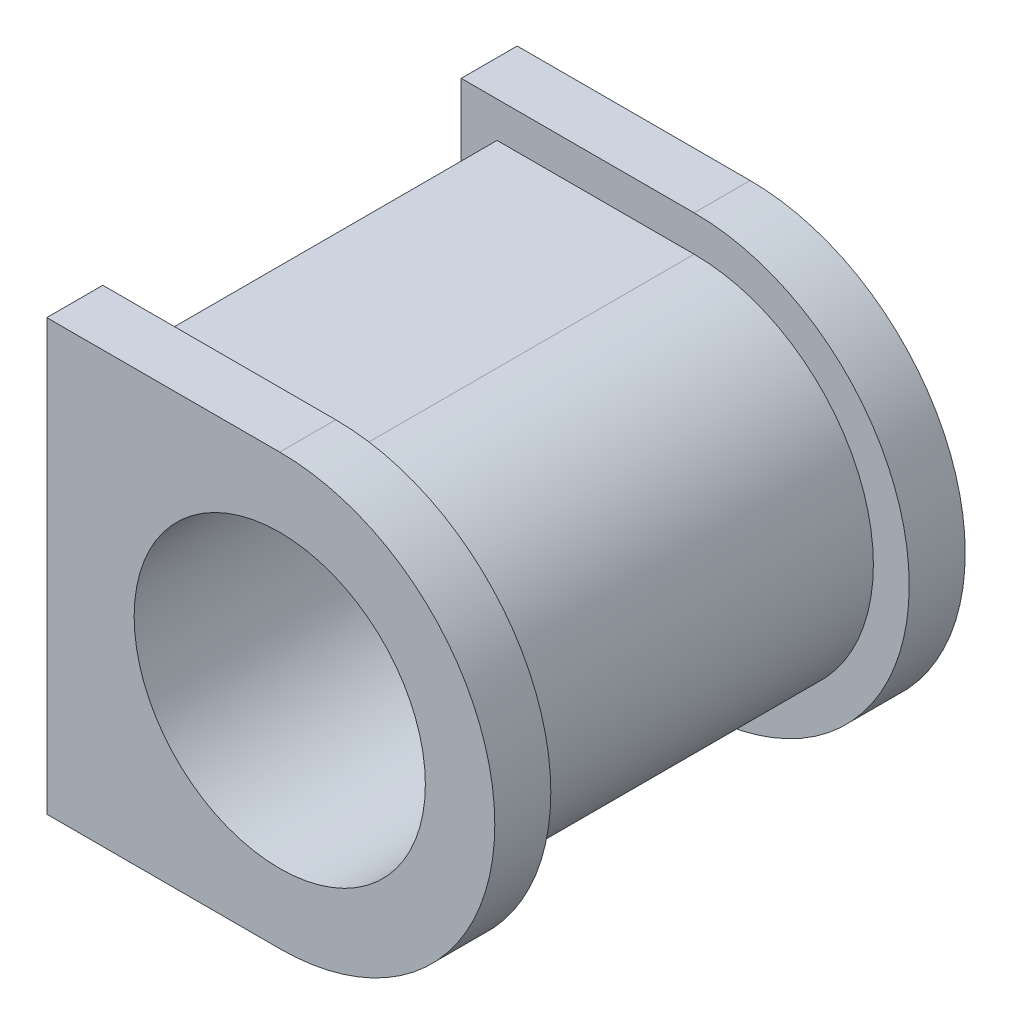
SolidWorks part; units mm, degrees
material "Alloy Steel"
ref_plane "Front Plane" through (0, 0, 0) normal (0, 0, 1) x (1, 0, 0)
ref_plane "Top Plane" through (0, 0, 0) normal (0, 1, 0) x (1, 0, 0)
ref_plane "Right Plane" through (0, 0, 0) normal (1, 0, 0) x (0, 0, -1)
sketch "Bush Profile Sketch" plane through (0, 0, 0) normal (0, 0, 1) x (1, 0, 0)
  line L0 (0, 40) -> (-44, 40)
  line L1 (0, -40) -> (-44, -40)
  line L2 (-44, -40) -> (-44, 40)
  circle A0 centre (0, 0) radius 32.5
  arc A1 (0, -40) -> (0, 40) centre (0, 0) ccw
  dimension "D1" = 65
  dimension "D2" = 80
  dimension "D3" = 44
extrude "Bush Body" add sketch "Bush Profile Sketch" along normal mid plane 80
sketch "Flange Profile Sketch" plane through (0, 0, 40) normal (0, 0, 1) x (1, 0, 0)
  line L1 (0, 48) -> (-52, 48)
  line L2 (-52, 48) -> (-52, -48)
  line L3 (-52, -48) -> (0, -48)
  arc A2 (0, -48) -> (0, 48) centre (0, 0) ccw
  arc A5 (0, -40) -> (0, 40) centre (0, 0) ccw construction
  circle A6 centre (0, 0) radius 32.5 construction
  circle A7 centre (0, 0) radius 32.5
  dimension "D1" = 96
  dimension "D2" = 52
extrude "End Flange" add sketch "Flange Profile Sketch" along normal blind 12.5
mirror "End Flange Mirror" about plane through (0, 0, 0) normal (0, 0, 1) of "End Flange"
